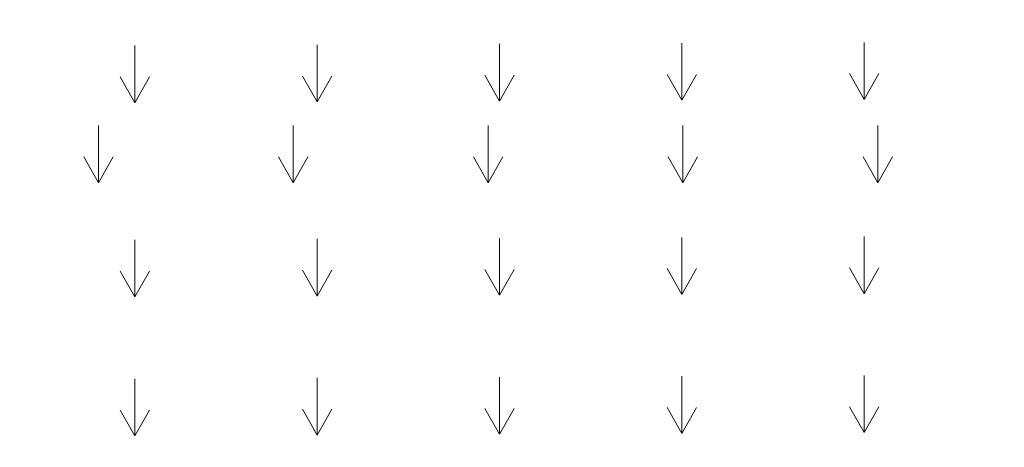
# Model space of a CAD drawing. Units: millimetres. Extents: x 595116 to 630915, y 909473 to 920225.
# Tile 41 of 134: x 629622 to 629682, y 919190 to 919216. Entities that reach past the tile are written whole.
import ezdxf

# ---------------------------------------------------------------- set-up
doc = ezdxf.new("R2010")
doc.units = ezdxf.units.MM
doc.layers.add('Dimension', color=3, linetype='Continuous', lineweight=18)
doc.layers.add('L-PLNT', color=85, linetype='Continuous', lineweight=13)
doc.styles.get("Standard").update_dxf_attribs({"font": 'arial.ttf'})
doc.dimstyles.new('ISO-25', dxfattribs={"dimtxt": 9, "dimasz": 6, "dimexe": 1.25, "dimexo": 0.625, "dimtad": 1, "dimlunit": 4, "dimtxsty": 'Standard', "dimcen": 2.5, "dimadec": 0, "dimazin": 0, "dimtfac": 1, "dimtmove": 0, "dimatfit": 3, "dimfxl": 1, "dimarcsym": 0})

# ---------------------------------------------------------------- blocks, each defined once
blk = doc.blocks.new('LAWN-GRASS-TUFT')
blk.add_line((0.892, 3.485), (0.892, 0))
blk.add_lwpolyline([(0, 1.577), (0.892, 0), (1.785, 1.577)])
blk = doc.blocks.new('*D216')
at = {"layer": 'Defpoints', "color": 0, "transparency": 16777216}
for p in [(629743.541, 919411.928), (629505.041, 919411.828), (629743.541, 918832.378)]:
    blk.add_point(p, dxfattribs=at)
at = {"layer": 'Dimension', "color": 0, "lineweight": -2, "transparency": 16777216}
for p, q in [((629505.041, 919411.203), (629505.041, 918831.128)), ((629743.541, 919411.303), (629743.541, 918831.128)), ((629511.041, 918832.378), (629737.541, 918832.378))]:
    blk.add_line(p, q, dxfattribs=at)
at = {"layer": 'Dimension', "color": 0, "transparency": 16777216}
for points in [[(629511.041, 918833.378), (629511.041, 918831.378), (629505.041, 918832.378)], [(629737.541, 918833.378), (629737.541, 918831.378), (629743.541, 918832.378)]]:
    blk.add_solid(points, dxfattribs=at)
at = {"layer": 'Dimension', "color": 0, "transparency": 16777216, "insert": (629624.291, 918837.656), "char_height": 9, "attachment_point": 5}
blk.add_mtext('19\'-10 1/2"', dxfattribs=at)

msp = doc.modelspace()

# ---------------------------------------------------------------- block references
at = {"layer": 'L-PLNT'}
for p in [(629628.026, 919211.325), (629639.139, 919211.374), (629650.253, 919211.424), (629661.367, 919211.474), (629672.481, 919211.523), (629625.811, 919206.447), (629637.684, 919206.447), (629649.557, 919206.447), (629661.43, 919206.447), (629673.303, 919206.447), (629672.481, 919199.685), (629628.026, 919199.487), (629639.139, 919199.536), (629650.253, 919199.586), (629661.367, 919199.635), (629628.026, 919191.017), (629639.139, 919191.067), (629650.253, 919191.116), (629661.367, 919191.166), (629672.481, 919191.215)]:
    msp.add_blockref('LAWN-GRASS-TUFT', p, dxfattribs=at)

# ---------------------------------------------------------------- dimensions: what is measured, and where the dimension line sits
at = {"layer": 'Dimension'}
dim = msp.add_linear_dim(base=(629743.541, 918832.378), p1=(629505.041, 919411.828), p2=(629743.541, 919411.928), dimstyle='ISO-25', override={"dimdec": 1, "dimlfac": 1, "dimrnd": 0, "dimzin": 1, "dimdsep": 46, "dimlunit": 4, "dimfrac": 2}, dxfattribs=at)
dim.commit()
dim.dimension.update_dxf_attribs({"geometry": '*D216', "text_midpoint": (629624.291, 918837.656)})

doc.saveas('drawing.dxf')
